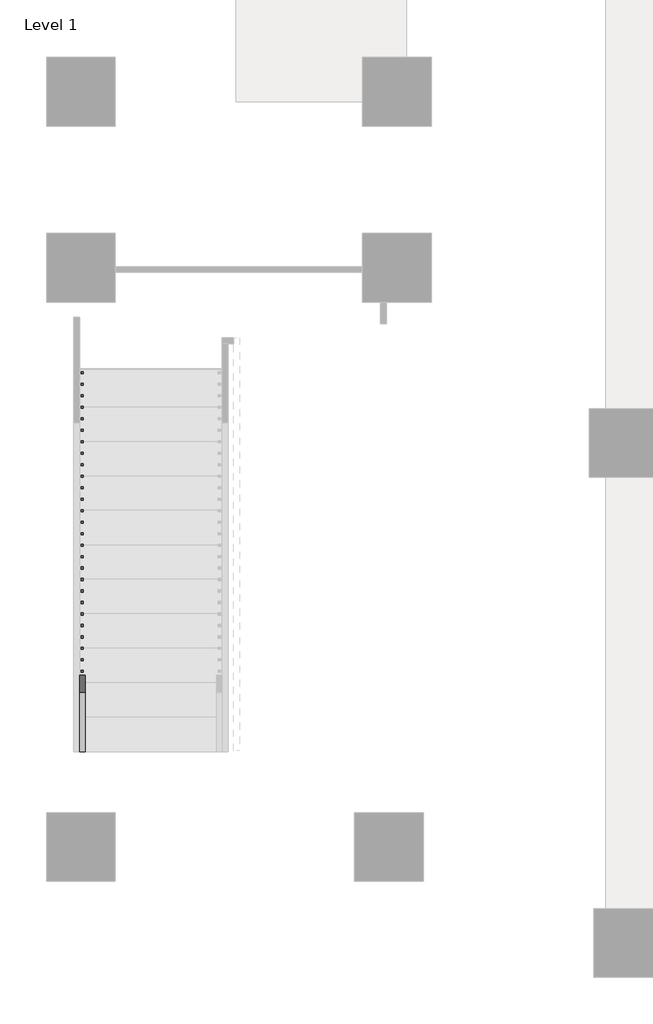
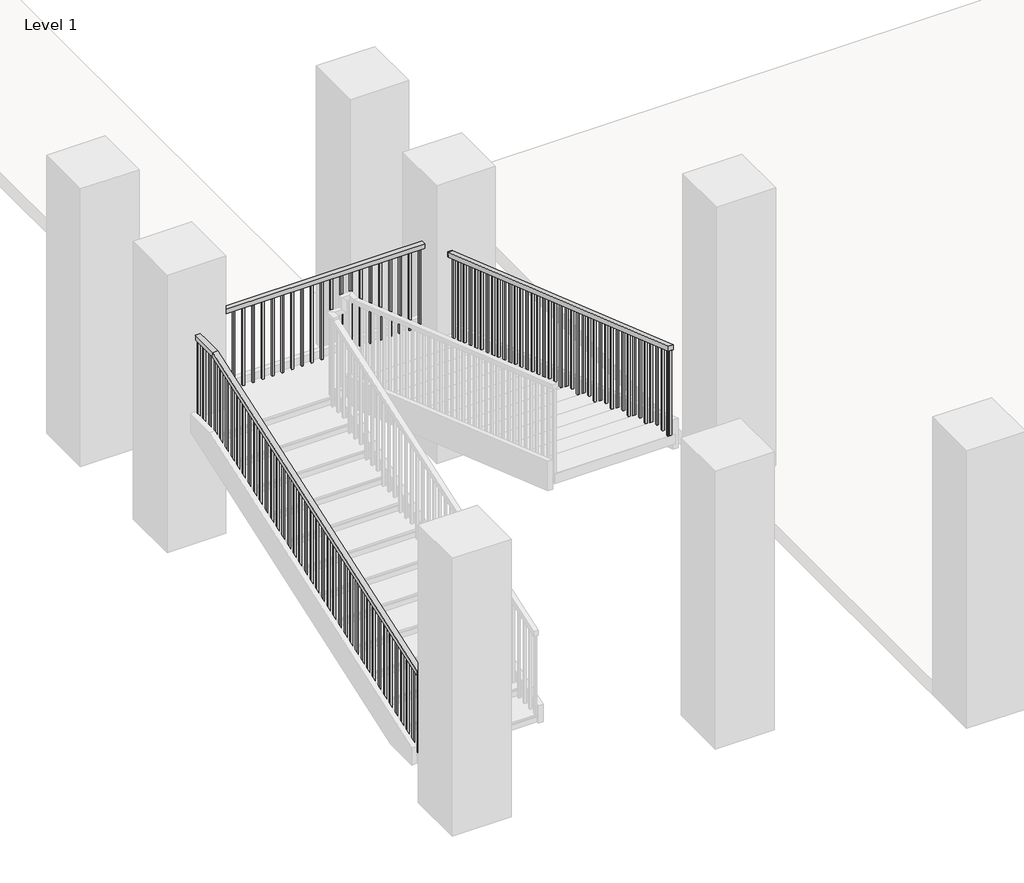
# One storey, part 4 of 6: 1 railing.
"""IFC4 building model written with IfcOpenShell, lengths in millimetres."""

from ifc_helpers import new_model, si_unit, frame, origin, place, context, project, spatial, polyline, outline, extrude, faceted_brep, element, save

model = new_model("IFC4")

# Units and contexts
model_context = context("Model", 3, world=origin())
ifc_project = project(units=[si_unit("LENGTHUNIT", "METRE", prefix="MILLI")], contexts=[model_context])

# Site, building, storey
site = spatial("IfcSite", under=ifc_project)
building = spatial("IfcBuilding", under=site)
storey = spatial("IfcBuildingStorey", under=building, Name="Level 1", Elevation=0.0)

# Railing
placement = place(None, origin())
element("IfcRailing", 1, ObjectType="Handrail - Rectangular", at=placement, inside=storey, context=model_context, shape_type="SolidModel", body=[
    faceted_brep([(-3857.687215, -9955.5916506, 1019.9076923), (-3857.687215, -9955.5916506, 966.1602476), (-3806.887215, -9955.5916506, 966.1602476), (-3806.887215, -9955.5916506, 1019.9076923), (-3857.687215, -6291.6416506, 2286.0), (-3857.687215, -6283.1120276, 2235.2), (-3806.887215, -6283.1120276, 2235.2), (-3806.887215, -6291.6416506, 2286.0), (-3857.687215, -5713.7916506, 2286.0), (-3857.687215, -5713.7916506, 2235.2), (-3806.887215, -5764.5916506, 2235.2), (-3806.887215, -5764.5916506, 2286.0), (-1190.687215, -5713.7916506, 2286.0), (-1190.687215, -5713.7916506, 2235.2), (-1241.487215, -5764.5916506, 2235.2), (-1241.487215, -5764.5916506, 2286.0), (-1190.687215, -5986.8416506, 2286.0), (-1190.687215, -5995.3852679, 2235.2), (-1241.487215, -5995.3852679, 2235.2), (-1241.487215, -5986.8416506, 2286.0), (-1190.687215, -9949.2416506, 3657.6), (-1241.487215, -9949.2416506, 3657.6), (-1241.487215, -9949.2416506, 3603.842594), (-1190.687215, -9949.2416506, 3603.842594)], [[[0, 1, 2, 3]], [[1, 0, 4, 5]], [[2, 1, 5, 6]], [[3, 2, 6, 7]], [[0, 3, 7, 4]], [[5, 4, 8, 9]], [[6, 5, 9, 10]], [[7, 6, 10, 11]], [[4, 7, 11, 8]], [[9, 8, 12, 13]], [[10, 9, 13, 14]], [[11, 10, 14, 15]], [[8, 11, 15, 12]], [[13, 12, 16, 17]], [[14, 13, 17, 18]], [[15, 14, 18, 19]], [[12, 15, 19, 16]], [[20, 21, 22, 23]], [[17, 16, 20, 23]], [[18, 17, 23, 22]], [[19, 18, 22, 21]], [[16, 19, 21, 20]]]),
    extrude(outline(polyline([(-9895.2666506, 3585.1589402), (-9895.2666506, 2637.6923077), (-9914.3166506, 2637.6923077), (-9914.3166506, 3591.7531709), (-9895.2666506, 3585.1589402)])), frame((-1225.612215, 0.0, 0.0), z_axis=(1.0, 0.0, 0.0), x_axis=(0.0, 1.0, 0.0)), (0.0, 0.0, 1.0), 19.05),
    extrude(outline(polyline([(-9793.6666506, 3549.9897094), (-9793.6666506, 2637.6923077), (-9812.7166506, 2637.6923077), (-9812.7166506, 3556.5839402), (-9793.6666506, 3549.9897094)])), frame((-1225.612215, 0.0, 0.0), z_axis=(1.0, 0.0, 0.0), x_axis=(0.0, 1.0, 0.0)), (0.0, 0.0, 1.0), 19.05),
    extrude(outline(polyline([(-9692.0666506, 3514.8204786), (-9692.0666506, 2637.6923077), (-9711.1166506, 2637.6923077), (-9711.1166506, 3521.4147094), (-9692.0666506, 3514.8204786)])), frame((-1225.612215, 0.0, 0.0), z_axis=(1.0, 0.0, 0.0), x_axis=(0.0, 1.0, 0.0)), (0.0, 0.0, 1.0), 19.05),
    extrude(outline(polyline([(-9590.4666506, 3479.6512479), (-9590.4666506, 2532.1846154), (-9609.5166506, 2532.1846154), (-9609.5166506, 3486.2454786), (-9590.4666506, 3479.6512479)])), frame((-1225.612215, 0.0, 0.0), z_axis=(1.0, 0.0, 0.0), x_axis=(0.0, 1.0, 0.0)), (0.0, 0.0, 1.0), 19.05),
    extrude(outline(polyline([(-9488.8666506, 3444.4820171), (-9488.8666506, 2532.1846154), (-9507.9166506, 2532.1846154), (-9507.9166506, 3451.0762479), (-9488.8666506, 3444.4820171)])), frame((-1225.612215, 0.0, 0.0), z_axis=(1.0, 0.0, 0.0), x_axis=(0.0, 1.0, 0.0)), (0.0, 0.0, 1.0), 19.05),
    extrude(outline(polyline([(-9387.2666506, 3409.3127863), (-9387.2666506, 2532.1846154), (-9406.3166506, 2532.1846154), (-9406.3166506, 3415.9070171), (-9387.2666506, 3409.3127863)])), frame((-1225.612215, 0.0, 0.0), z_axis=(1.0, 0.0, 0.0), x_axis=(0.0, 1.0, 0.0)), (0.0, 0.0, 1.0), 19.05),
    extrude(outline(polyline([(-9285.6666506, 3374.1435556), (-9285.6666506, 2426.6769231), (-9304.7166506, 2426.6769231), (-9304.7166506, 3380.7377863), (-9285.6666506, 3374.1435556)])), frame((-1225.612215, 0.0, 0.0), z_axis=(1.0, 0.0, 0.0), x_axis=(0.0, 1.0, 0.0)), (0.0, 0.0, 1.0), 19.05),
    extrude(outline(polyline([(-9184.0666506, 3338.9743248), (-9184.0666506, 2426.6769231), (-9203.1166506, 2426.6769231), (-9203.1166506, 3345.5685556), (-9184.0666506, 3338.9743248)])), frame((-1225.612215, 0.0, 0.0), z_axis=(1.0, 0.0, 0.0), x_axis=(0.0, 1.0, 0.0)), (0.0, 0.0, 1.0), 19.05),
    extrude(outline(polyline([(-9082.4666506, 3303.805094), (-9082.4666506, 2426.6769231), (-9101.5166506, 2426.6769231), (-9101.5166506, 3310.3993248), (-9082.4666506, 3303.805094)])), frame((-1225.612215, 0.0, 0.0), z_axis=(1.0, 0.0, 0.0), x_axis=(0.0, 1.0, 0.0)), (0.0, 0.0, 1.0), 19.05),
    extrude(outline(polyline([(-8980.8666506, 3268.6358632), (-8980.8666506, 2321.1692308), (-8999.9166506, 2321.1692308), (-8999.9166506, 3275.230094), (-8980.8666506, 3268.6358632)])), frame((-1225.612215, 0.0, 0.0), z_axis=(1.0, 0.0, 0.0), x_axis=(0.0, 1.0, 0.0)), (0.0, 0.0, 1.0), 19.05),
    extrude(outline(polyline([(-8879.2666506, 3233.4666325), (-8879.2666506, 2321.1692308), (-8898.3166506, 2321.1692308), (-8898.3166506, 3240.0608632), (-8879.2666506, 3233.4666325)])), frame((-1225.612215, 0.0, 0.0), z_axis=(1.0, 0.0, 0.0), x_axis=(0.0, 1.0, 0.0)), (0.0, 0.0, 1.0), 19.05),
    extrude(outline(polyline([(-8777.6666506, 3198.2974017), (-8777.6666506, 2321.1692308), (-8796.7166506, 2321.1692308), (-8796.7166506, 3204.8916325), (-8777.6666506, 3198.2974017)])), frame((-1225.612215, 0.0, 0.0), z_axis=(1.0, 0.0, 0.0), x_axis=(0.0, 1.0, 0.0)), (0.0, 0.0, 1.0), 19.05),
    extrude(outline(polyline([(-8676.0666506, 3163.1281709), (-8676.0666506, 2215.6615385), (-8695.1166506, 2215.6615385), (-8695.1166506, 3169.7224017), (-8676.0666506, 3163.1281709)])), frame((-1225.612215, 0.0, 0.0), z_axis=(1.0, 0.0, 0.0), x_axis=(0.0, 1.0, 0.0)), (0.0, 0.0, 1.0), 19.05),
    extrude(outline(polyline([(-8574.4666506, 3127.9589402), (-8574.4666506, 2215.6615385), (-8593.5166506, 2215.6615385), (-8593.5166506, 3134.5531709), (-8574.4666506, 3127.9589402)])), frame((-1225.612215, 0.0, 0.0), z_axis=(1.0, 0.0, 0.0), x_axis=(0.0, 1.0, 0.0)), (0.0, 0.0, 1.0), 19.05),
    extrude(outline(polyline([(-8472.8666506, 3092.7897094), (-8472.8666506, 2215.6615385), (-8491.9166506, 2215.6615385), (-8491.9166506, 3099.3839402), (-8472.8666506, 3092.7897094)])), frame((-1225.612215, 0.0, 0.0), z_axis=(1.0, 0.0, 0.0), x_axis=(0.0, 1.0, 0.0)), (0.0, 0.0, 1.0), 19.05),
    extrude(outline(polyline([(-8371.2666506, 3057.6204786), (-8371.2666506, 2110.1538462), (-8390.3166506, 2110.1538462), (-8390.3166506, 3064.2147094), (-8371.2666506, 3057.6204786)])), frame((-1225.612215, 0.0, 0.0), z_axis=(1.0, 0.0, 0.0), x_axis=(0.0, 1.0, 0.0)), (0.0, 0.0, 1.0), 19.05),
    extrude(outline(polyline([(-8269.6666506, 3022.4512479), (-8269.6666506, 2110.1538462), (-8288.7166506, 2110.1538462), (-8288.7166506, 3029.0454786), (-8269.6666506, 3022.4512479)])), frame((-1225.612215, 0.0, 0.0), z_axis=(1.0, 0.0, 0.0), x_axis=(0.0, 1.0, 0.0)), (0.0, 0.0, 1.0), 19.05),
    extrude(outline(polyline([(-8168.0666506, 2987.2820171), (-8168.0666506, 2110.1538462), (-8187.1166506, 2110.1538462), (-8187.1166506, 2993.8762479), (-8168.0666506, 2987.2820171)])), frame((-1225.612215, 0.0, 0.0), z_axis=(1.0, 0.0, 0.0), x_axis=(0.0, 1.0, 0.0)), (0.0, 0.0, 1.0), 19.05),
    extrude(outline(polyline([(-8066.4666506, 2952.1127863), (-8066.4666506, 2004.6461538), (-8085.5166506, 2004.6461538), (-8085.5166506, 2958.7070171), (-8066.4666506, 2952.1127863)])), frame((-1225.612215, 0.0, 0.0), z_axis=(1.0, 0.0, 0.0), x_axis=(0.0, 1.0, 0.0)), (0.0, 0.0, 1.0), 19.05),
    extrude(outline(polyline([(-7964.8666506, 2916.9435556), (-7964.8666506, 2004.6461538), (-7983.9166506, 2004.6461538), (-7983.9166506, 2923.5377863), (-7964.8666506, 2916.9435556)])), frame((-1225.612215, 0.0, 0.0), z_axis=(1.0, 0.0, 0.0), x_axis=(0.0, 1.0, 0.0)), (0.0, 0.0, 1.0), 19.05),
    extrude(outline(polyline([(-7863.2666506, 2881.7743248), (-7863.2666506, 2004.6461538), (-7882.3166506, 2004.6461538), (-7882.3166506, 2888.3685556), (-7863.2666506, 2881.7743248)])), frame((-1225.612215, 0.0, 0.0), z_axis=(1.0, 0.0, 0.0), x_axis=(0.0, 1.0, 0.0)), (0.0, 0.0, 1.0), 19.05),
    extrude(outline(polyline([(-7761.6666506, 2846.605094), (-7761.6666506, 1899.1384615), (-7780.7166506, 1899.1384615), (-7780.7166506, 2853.1993248), (-7761.6666506, 2846.605094)])), frame((-1225.612215, 0.0, 0.0), z_axis=(1.0, 0.0, 0.0), x_axis=(0.0, 1.0, 0.0)), (0.0, 0.0, 1.0), 19.05),
    extrude(outline(polyline([(-7660.0666506, 2811.4358632), (-7660.0666506, 1899.1384615), (-7679.1166506, 1899.1384615), (-7679.1166506, 2818.030094), (-7660.0666506, 2811.4358632)])), frame((-1225.612215, 0.0, 0.0), z_axis=(1.0, 0.0, 0.0), x_axis=(0.0, 1.0, 0.0)), (0.0, 0.0, 1.0), 19.05),
    extrude(outline(polyline([(-7558.4666506, 2776.2666325), (-7558.4666506, 1899.1384615), (-7577.5166506, 1899.1384615), (-7577.5166506, 2782.8608632), (-7558.4666506, 2776.2666325)])), frame((-1225.612215, 0.0, 0.0), z_axis=(1.0, 0.0, 0.0), x_axis=(0.0, 1.0, 0.0)), (0.0, 0.0, 1.0), 19.05),
    extrude(outline(polyline([(-7456.8666506, 2741.0974017), (-7456.8666506, 1793.6307692), (-7475.9166506, 1793.6307692), (-7475.9166506, 2747.6916325), (-7456.8666506, 2741.0974017)])), frame((-1225.612215, 0.0, 0.0), z_axis=(1.0, 0.0, 0.0), x_axis=(0.0, 1.0, 0.0)), (0.0, 0.0, 1.0), 19.05),
    extrude(outline(polyline([(-7355.2666506, 2705.9281709), (-7355.2666506, 1793.6307692), (-7374.3166506, 1793.6307692), (-7374.3166506, 2712.5224017), (-7355.2666506, 2705.9281709)])), frame((-1225.612215, 0.0, 0.0), z_axis=(1.0, 0.0, 0.0), x_axis=(0.0, 1.0, 0.0)), (0.0, 0.0, 1.0), 19.05),
    extrude(outline(polyline([(-7253.6666506, 2670.7589402), (-7253.6666506, 1793.6307692), (-7272.7166506, 1793.6307692), (-7272.7166506, 2677.3531709), (-7253.6666506, 2670.7589402)])), frame((-1225.612215, 0.0, 0.0), z_axis=(1.0, 0.0, 0.0), x_axis=(0.0, 1.0, 0.0)), (0.0, 0.0, 1.0), 19.05),
    extrude(outline(polyline([(-7152.0666506, 2635.5897094), (-7152.0666506, 1688.1230769), (-7171.1166506, 1688.1230769), (-7171.1166506, 2642.1839402), (-7152.0666506, 2635.5897094)])), frame((-1225.612215, 0.0, 0.0), z_axis=(1.0, 0.0, 0.0), x_axis=(0.0, 1.0, 0.0)), (0.0, 0.0, 1.0), 19.05),
    extrude(outline(polyline([(-7050.4666506, 2600.4204786), (-7050.4666506, 1688.1230769), (-7069.5166506, 1688.1230769), (-7069.5166506, 2607.0147094), (-7050.4666506, 2600.4204786)])), frame((-1225.612215, 0.0, 0.0), z_axis=(1.0, 0.0, 0.0), x_axis=(0.0, 1.0, 0.0)), (0.0, 0.0, 1.0), 19.05),
    extrude(outline(polyline([(-6948.8666506, 2565.2512479), (-6948.8666506, 1688.1230769), (-6967.9166506, 1688.1230769), (-6967.9166506, 2571.8454786), (-6948.8666506, 2565.2512479)])), frame((-1225.612215, 0.0, 0.0), z_axis=(1.0, 0.0, 0.0), x_axis=(0.0, 1.0, 0.0)), (0.0, 0.0, 1.0), 19.05),
    extrude(outline(polyline([(-6847.2666506, 2530.0820171), (-6847.2666506, 1582.6153846), (-6866.3166506, 1582.6153846), (-6866.3166506, 2536.6762479), (-6847.2666506, 2530.0820171)])), frame((-1225.612215, 0.0, 0.0), z_axis=(1.0, 0.0, 0.0), x_axis=(0.0, 1.0, 0.0)), (0.0, 0.0, 1.0), 19.05),
    extrude(outline(polyline([(-6745.6666506, 2494.9127863), (-6745.6666506, 1582.6153846), (-6764.7166506, 1582.6153846), (-6764.7166506, 2501.5070171), (-6745.6666506, 2494.9127863)])), frame((-1225.612215, 0.0, 0.0), z_axis=(1.0, 0.0, 0.0), x_axis=(0.0, 1.0, 0.0)), (0.0, 0.0, 1.0), 19.05),
    extrude(outline(polyline([(-6644.0666506, 2459.7435556), (-6644.0666506, 1582.6153846), (-6663.1166506, 1582.6153846), (-6663.1166506, 2466.3377863), (-6644.0666506, 2459.7435556)])), frame((-1225.612215, 0.0, 0.0), z_axis=(1.0, 0.0, 0.0), x_axis=(0.0, 1.0, 0.0)), (0.0, 0.0, 1.0), 19.05),
    extrude(outline(polyline([(-6542.4666506, 2424.5743248), (-6542.4666506, 1477.1076923), (-6561.5166506, 1477.1076923), (-6561.5166506, 2431.1685556), (-6542.4666506, 2424.5743248)])), frame((-1225.612215, 0.0, 0.0), z_axis=(1.0, 0.0, 0.0), x_axis=(0.0, 1.0, 0.0)), (0.0, 0.0, 1.0), 19.05),
    extrude(outline(polyline([(-6440.8666506, 2389.405094), (-6440.8666506, 1477.1076923), (-6459.9166506, 1477.1076923), (-6459.9166506, 2395.9993248), (-6440.8666506, 2389.405094)])), frame((-1225.612215, 0.0, 0.0), z_axis=(1.0, 0.0, 0.0), x_axis=(0.0, 1.0, 0.0)), (0.0, 0.0, 1.0), 19.05),
    extrude(outline(polyline([(-6339.2666506, 2354.2358632), (-6339.2666506, 1477.1076923), (-6358.3166506, 1477.1076923), (-6358.3166506, 2360.830094), (-6339.2666506, 2354.2358632)])), frame((-1225.612215, 0.0, 0.0), z_axis=(1.0, 0.0, 0.0), x_axis=(0.0, 1.0, 0.0)), (0.0, 0.0, 1.0), 19.05),
    extrude(outline(polyline([(-6237.6666506, 2319.0666325), (-6237.6666506, 1371.6), (-6256.7166506, 1371.6), (-6256.7166506, 2325.6608632), (-6237.6666506, 2319.0666325)])), frame((-1225.612215, 0.0, 0.0), z_axis=(1.0, 0.0, 0.0), x_axis=(0.0, 1.0, 0.0)), (0.0, 0.0, 1.0), 19.05),
    extrude(outline(polyline([(-6136.0666506, 2283.8974017), (-6136.0666506, 1371.6), (-6155.1166506, 1371.6), (-6155.1166506, 2290.4916325), (-6136.0666506, 2283.8974017)])), frame((-1225.612215, 0.0, 0.0), z_axis=(1.0, 0.0, 0.0), x_axis=(0.0, 1.0, 0.0)), (0.0, 0.0, 1.0), 19.05),
    extrude(outline(polyline([(-6034.4666506, 2248.7281709), (-6034.4666506, 1371.6), (-6053.5166506, 1371.6), (-6053.5166506, 2255.3224017), (-6034.4666506, 2248.7281709)])), frame((-1225.612215, 0.0, 0.0), z_axis=(1.0, 0.0, 0.0), x_axis=(0.0, 1.0, 0.0)), (0.0, 0.0, 1.0), 19.05),
    extrude(outline(polyline([(-1206.562215, -5932.8666506), (-1206.562215, -5951.9166506), (-1225.612215, -5951.9166506), (-1225.612215, -5932.8666506), (-1206.562215, -5932.8666506)])), frame((0.0, 0.0, 1371.6), z_axis=(0.0, 0.0, 1.0), x_axis=(1.0, 0.0, 0.0)), (0.0, 0.0, 1.0), 863.6),
    extrude(outline(polyline([(-1206.562215, -5831.2666506), (-1206.562215, -5850.3166506), (-1225.612215, -5850.3166506), (-1225.612215, -5831.2666506), (-1206.562215, -5831.2666506)])), frame((0.0, 0.0, 1371.6), z_axis=(0.0, 0.0, 1.0), x_axis=(1.0, 0.0, 0.0)), (0.0, 0.0, 1.0), 863.6),
    extrude(outline(polyline([(-1301.812215, -5729.6666506), (-1282.762215, -5729.6666506), (-1282.762215, -5748.7166506), (-1301.812215, -5748.7166506), (-1301.812215, -5729.6666506)])), frame((0.0, 0.0, 1371.6), z_axis=(0.0, 0.0, 1.0), x_axis=(1.0, 0.0, 0.0)), (0.0, 0.0, 1.0), 863.6),
    extrude(outline(polyline([(-1403.412215, -5729.6666506), (-1384.362215, -5729.6666506), (-1384.362215, -5748.7166506), (-1403.412215, -5748.7166506), (-1403.412215, -5729.6666506)])), frame((0.0, 0.0, 1371.6), z_axis=(0.0, 0.0, 1.0), x_axis=(1.0, 0.0, 0.0)), (0.0, 0.0, 1.0), 863.6),
    extrude(outline(polyline([(-1505.012215, -5729.6666506), (-1485.962215, -5729.6666506), (-1485.962215, -5748.7166506), (-1505.012215, -5748.7166506), (-1505.012215, -5729.6666506)])), frame((0.0, 0.0, 1371.6), z_axis=(0.0, 0.0, 1.0), x_axis=(1.0, 0.0, 0.0)), (0.0, 0.0, 1.0), 863.6),
    extrude(outline(polyline([(-1606.612215, -5729.6666506), (-1587.562215, -5729.6666506), (-1587.562215, -5748.7166506), (-1606.612215, -5748.7166506), (-1606.612215, -5729.6666506)])), frame((0.0, 0.0, 1371.6), z_axis=(0.0, 0.0, 1.0), x_axis=(1.0, 0.0, 0.0)), (0.0, 0.0, 1.0), 863.6),
    extrude(outline(polyline([(-1708.212215, -5729.6666506), (-1689.162215, -5729.6666506), (-1689.162215, -5748.7166506), (-1708.212215, -5748.7166506), (-1708.212215, -5729.6666506)])), frame((0.0, 0.0, 1371.6), z_axis=(0.0, 0.0, 1.0), x_axis=(1.0, 0.0, 0.0)), (0.0, 0.0, 1.0), 863.6),
    extrude(outline(polyline([(-1809.812215, -5729.6666506), (-1790.762215, -5729.6666506), (-1790.762215, -5748.7166506), (-1809.812215, -5748.7166506), (-1809.812215, -5729.6666506)])), frame((0.0, 0.0, 1371.6), z_axis=(0.0, 0.0, 1.0), x_axis=(1.0, 0.0, 0.0)), (0.0, 0.0, 1.0), 863.6),
    extrude(outline(polyline([(-1911.412215, -5729.6666506), (-1892.362215, -5729.6666506), (-1892.362215, -5748.7166506), (-1911.412215, -5748.7166506), (-1911.412215, -5729.6666506)])), frame((0.0, 0.0, 1371.6), z_axis=(0.0, 0.0, 1.0), x_axis=(1.0, 0.0, 0.0)), (0.0, 0.0, 1.0), 863.6),
    extrude(outline(polyline([(-2013.012215, -5729.6666506), (-1993.962215, -5729.6666506), (-1993.962215, -5748.7166506), (-2013.012215, -5748.7166506), (-2013.012215, -5729.6666506)])), frame((0.0, 0.0, 1371.6), z_axis=(0.0, 0.0, 1.0), x_axis=(1.0, 0.0, 0.0)), (0.0, 0.0, 1.0), 863.6),
    extrude(outline(polyline([(-2114.612215, -5729.6666506), (-2095.562215, -5729.6666506), (-2095.562215, -5748.7166506), (-2114.612215, -5748.7166506), (-2114.612215, -5729.6666506)])), frame((0.0, 0.0, 1371.6), z_axis=(0.0, 0.0, 1.0), x_axis=(1.0, 0.0, 0.0)), (0.0, 0.0, 1.0), 863.6),
    extrude(outline(polyline([(-2216.212215, -5729.6666506), (-2197.162215, -5729.6666506), (-2197.162215, -5748.7166506), (-2216.212215, -5748.7166506), (-2216.212215, -5729.6666506)])), frame((0.0, 0.0, 1371.6), z_axis=(0.0, 0.0, 1.0), x_axis=(1.0, 0.0, 0.0)), (0.0, 0.0, 1.0), 863.6),
    extrude(outline(polyline([(-2317.812215, -5729.6666506), (-2298.762215, -5729.6666506), (-2298.762215, -5748.7166506), (-2317.812215, -5748.7166506), (-2317.812215, -5729.6666506)])), frame((0.0, 0.0, 1371.6), z_axis=(0.0, 0.0, 1.0), x_axis=(1.0, 0.0, 0.0)), (0.0, 0.0, 1.0), 863.6),
    extrude(outline(polyline([(-2419.412215, -5729.6666506), (-2400.362215, -5729.6666506), (-2400.362215, -5748.7166506), (-2419.412215, -5748.7166506), (-2419.412215, -5729.6666506)])), frame((0.0, 0.0, 1371.6), z_axis=(0.0, 0.0, 1.0), x_axis=(1.0, 0.0, 0.0)), (0.0, 0.0, 1.0), 863.6),
    extrude(outline(polyline([(-2521.012215, -5729.6666506), (-2501.962215, -5729.6666506), (-2501.962215, -5748.7166506), (-2521.012215, -5748.7166506), (-2521.012215, -5729.6666506)])), frame((0.0, 0.0, 1371.6), z_axis=(0.0, 0.0, 1.0), x_axis=(1.0, 0.0, 0.0)), (0.0, 0.0, 1.0), 863.6),
    extrude(outline(polyline([(-2622.612215, -5729.6666506), (-2603.562215, -5729.6666506), (-2603.562215, -5748.7166506), (-2622.612215, -5748.7166506), (-2622.612215, -5729.6666506)])), frame((0.0, 0.0, 1371.6), z_axis=(0.0, 0.0, 1.0), x_axis=(1.0, 0.0, 0.0)), (0.0, 0.0, 1.0), 863.6),
    extrude(outline(polyline([(-2724.212215, -5729.6666506), (-2705.162215, -5729.6666506), (-2705.162215, -5748.7166506), (-2724.212215, -5748.7166506), (-2724.212215, -5729.6666506)])), frame((0.0, 0.0, 1371.6), z_axis=(0.0, 0.0, 1.0), x_axis=(1.0, 0.0, 0.0)), (0.0, 0.0, 1.0), 863.6),
    extrude(outline(polyline([(-2825.812215, -5729.6666506), (-2806.762215, -5729.6666506), (-2806.762215, -5748.7166506), (-2825.812215, -5748.7166506), (-2825.812215, -5729.6666506)])), frame((0.0, 0.0, 1371.6), z_axis=(0.0, 0.0, 1.0), x_axis=(1.0, 0.0, 0.0)), (0.0, 0.0, 1.0), 863.6),
    extrude(outline(polyline([(-2927.412215, -5729.6666506), (-2908.362215, -5729.6666506), (-2908.362215, -5748.7166506), (-2927.412215, -5748.7166506), (-2927.412215, -5729.6666506)])), frame((0.0, 0.0, 1371.6), z_axis=(0.0, 0.0, 1.0), x_axis=(1.0, 0.0, 0.0)), (0.0, 0.0, 1.0), 863.6),
    extrude(outline(polyline([(-3029.012215, -5729.6666506), (-3009.962215, -5729.6666506), (-3009.962215, -5748.7166506), (-3029.012215, -5748.7166506), (-3029.012215, -5729.6666506)])), frame((0.0, 0.0, 1371.6), z_axis=(0.0, 0.0, 1.0), x_axis=(1.0, 0.0, 0.0)), (0.0, 0.0, 1.0), 863.6),
    extrude(outline(polyline([(-3130.612215, -5729.6666506), (-3111.562215, -5729.6666506), (-3111.562215, -5748.7166506), (-3130.612215, -5748.7166506), (-3130.612215, -5729.6666506)])), frame((0.0, 0.0, 1371.6), z_axis=(0.0, 0.0, 1.0), x_axis=(1.0, 0.0, 0.0)), (0.0, 0.0, 1.0), 863.6),
    extrude(outline(polyline([(-3232.212215, -5729.6666506), (-3213.162215, -5729.6666506), (-3213.162215, -5748.7166506), (-3232.212215, -5748.7166506), (-3232.212215, -5729.6666506)])), frame((0.0, 0.0, 1371.6), z_axis=(0.0, 0.0, 1.0), x_axis=(1.0, 0.0, 0.0)), (0.0, 0.0, 1.0), 863.6),
    extrude(outline(polyline([(-3333.812215, -5729.6666506), (-3314.762215, -5729.6666506), (-3314.762215, -5748.7166506), (-3333.812215, -5748.7166506), (-3333.812215, -5729.6666506)])), frame((0.0, 0.0, 1371.6), z_axis=(0.0, 0.0, 1.0), x_axis=(1.0, 0.0, 0.0)), (0.0, 0.0, 1.0), 863.6),
    extrude(outline(polyline([(-3435.412215, -5729.6666506), (-3416.362215, -5729.6666506), (-3416.362215, -5748.7166506), (-3435.412215, -5748.7166506), (-3435.412215, -5729.6666506)])), frame((0.0, 0.0, 1371.6), z_axis=(0.0, 0.0, 1.0), x_axis=(1.0, 0.0, 0.0)), (0.0, 0.0, 1.0), 863.6),
    extrude(outline(polyline([(-3537.012215, -5729.6666506), (-3517.962215, -5729.6666506), (-3517.962215, -5748.7166506), (-3537.012215, -5748.7166506), (-3537.012215, -5729.6666506)])), frame((0.0, 0.0, 1371.6), z_axis=(0.0, 0.0, 1.0), x_axis=(1.0, 0.0, 0.0)), (0.0, 0.0, 1.0), 863.6),
    extrude(outline(polyline([(-3638.612215, -5729.6666506), (-3619.562215, -5729.6666506), (-3619.562215, -5748.7166506), (-3638.612215, -5748.7166506), (-3638.612215, -5729.6666506)])), frame((0.0, 0.0, 1371.6), z_axis=(0.0, 0.0, 1.0), x_axis=(1.0, 0.0, 0.0)), (0.0, 0.0, 1.0), 863.6),
    extrude(outline(polyline([(-3740.212215, -5729.6666506), (-3721.162215, -5729.6666506), (-3721.162215, -5748.7166506), (-3740.212215, -5748.7166506), (-3740.212215, -5729.6666506)])), frame((0.0, 0.0, 1371.6), z_axis=(0.0, 0.0, 1.0), x_axis=(1.0, 0.0, 0.0)), (0.0, 0.0, 1.0), 863.6),
    extrude(outline(polyline([(-3841.812215, -5799.5166506), (-3841.812215, -5780.4666506), (-3822.762215, -5780.4666506), (-3822.762215, -5799.5166506), (-3841.812215, -5799.5166506)])), frame((0.0, 0.0, 1371.6), z_axis=(0.0, 0.0, 1.0), x_axis=(1.0, 0.0, 0.0)), (0.0, 0.0, 1.0), 863.6),
    extrude(outline(polyline([(-3841.812215, -5901.1166506), (-3841.812215, -5882.0666506), (-3822.762215, -5882.0666506), (-3822.762215, -5901.1166506), (-3841.812215, -5901.1166506)])), frame((0.0, 0.0, 1371.6), z_axis=(0.0, 0.0, 1.0), x_axis=(1.0, 0.0, 0.0)), (0.0, 0.0, 1.0), 863.6),
    extrude(outline(polyline([(-3841.812215, -6002.7166506), (-3841.812215, -5983.6666506), (-3822.762215, -5983.6666506), (-3822.762215, -6002.7166506), (-3841.812215, -6002.7166506)])), frame((0.0, 0.0, 1371.6), z_axis=(0.0, 0.0, 1.0), x_axis=(1.0, 0.0, 0.0)), (0.0, 0.0, 1.0), 863.6),
    extrude(outline(polyline([(-3841.812215, -6104.3166506), (-3841.812215, -6085.2666506), (-3822.762215, -6085.2666506), (-3822.762215, -6104.3166506), (-3841.812215, -6104.3166506)])), frame((0.0, 0.0, 1371.6), z_axis=(0.0, 0.0, 1.0), x_axis=(1.0, 0.0, 0.0)), (0.0, 0.0, 1.0), 863.6),
    extrude(outline(polyline([(-3841.812215, -6205.9166506), (-3841.812215, -6186.8666506), (-3822.762215, -6186.8666506), (-3822.762215, -6205.9166506), (-3841.812215, -6205.9166506)])), frame((0.0, 0.0, 1371.6), z_axis=(0.0, 0.0, 1.0), x_axis=(1.0, 0.0, 0.0)), (0.0, 0.0, 1.0), 863.6),
    extrude(outline(polyline([(-6288.4666506, 2233.349689), (-6288.4666506, 1266.0923077), (-6307.5166506, 1266.0923077), (-6307.5166506, 2226.7668867), (-6288.4666506, 2233.349689)])), frame((-3841.812215, 0.0, 0.0), z_axis=(1.0, 0.0, 0.0), x_axis=(0.0, 1.0, 0.0)), (0.0, 0.0, 1.0), 19.05),
    extrude(outline(polyline([(-6390.0666506, 2198.2414101), (-6390.0666506, 1266.0923077), (-6409.1166506, 1266.0923077), (-6409.1166506, 2191.6586078), (-6390.0666506, 2198.2414101)])), frame((-3841.812215, 0.0, 0.0), z_axis=(1.0, 0.0, 0.0), x_axis=(0.0, 1.0, 0.0)), (0.0, 0.0, 1.0), 19.05),
    extrude(outline(polyline([(-6491.6666506, 2163.1331312), (-6491.6666506, 1266.0923077), (-6510.7166506, 1266.0923077), (-6510.7166506, 2156.5503289), (-6491.6666506, 2163.1331312)])), frame((-3841.812215, 0.0, 0.0), z_axis=(1.0, 0.0, 0.0), x_axis=(0.0, 1.0, 0.0)), (0.0, 0.0, 1.0), 19.05),
    extrude(outline(polyline([(-6593.2666506, 2128.0248523), (-6593.2666506, 1160.5846154), (-6612.3166506, 1160.5846154), (-6612.3166506, 2121.44205), (-6593.2666506, 2128.0248523)])), frame((-3841.812215, 0.0, 0.0), z_axis=(1.0, 0.0, 0.0), x_axis=(0.0, 1.0, 0.0)), (0.0, 0.0, 1.0), 19.05),
    extrude(outline(polyline([(-6694.8666506, 2092.9165734), (-6694.8666506, 1160.5846154), (-6713.9166506, 1160.5846154), (-6713.9166506, 2086.3337711), (-6694.8666506, 2092.9165734)])), frame((-3841.812215, 0.0, 0.0), z_axis=(1.0, 0.0, 0.0), x_axis=(0.0, 1.0, 0.0)), (0.0, 0.0, 1.0), 19.05),
    extrude(outline(polyline([(-6796.4666506, 2057.8082945), (-6796.4666506, 1160.5846154), (-6815.5166506, 1160.5846154), (-6815.5166506, 2051.2254922), (-6796.4666506, 2057.8082945)])), frame((-3841.812215, 0.0, 0.0), z_axis=(1.0, 0.0, 0.0), x_axis=(0.0, 1.0, 0.0)), (0.0, 0.0, 1.0), 19.05),
    extrude(outline(polyline([(-6898.0666506, 2022.7000156), (-6898.0666506, 1055.0769231), (-6917.1166506, 1055.0769231), (-6917.1166506, 2016.1172133), (-6898.0666506, 2022.7000156)])), frame((-3841.812215, 0.0, 0.0), z_axis=(1.0, 0.0, 0.0), x_axis=(0.0, 1.0, 0.0)), (0.0, 0.0, 1.0), 19.05),
    extrude(outline(polyline([(-6999.6666506, 1987.5917367), (-6999.6666506, 1055.0769231), (-7018.7166506, 1055.0769231), (-7018.7166506, 1981.0089344), (-6999.6666506, 1987.5917367)])), frame((-3841.812215, 0.0, 0.0), z_axis=(1.0, 0.0, 0.0), x_axis=(0.0, 1.0, 0.0)), (0.0, 0.0, 1.0), 19.05),
    extrude(outline(polyline([(-7101.2666506, 1952.4834578), (-7101.2666506, 1055.0769231), (-7120.3166506, 1055.0769231), (-7120.3166506, 1945.9006556), (-7101.2666506, 1952.4834578)])), frame((-3841.812215, 0.0, 0.0), z_axis=(1.0, 0.0, 0.0), x_axis=(0.0, 1.0, 0.0)), (0.0, 0.0, 1.0), 19.05),
    extrude(outline(polyline([(-7202.8666506, 1917.375179), (-7202.8666506, 949.5692308), (-7221.9166506, 949.5692308), (-7221.9166506, 1910.7923767), (-7202.8666506, 1917.375179)])), frame((-3841.812215, 0.0, 0.0), z_axis=(1.0, 0.0, 0.0), x_axis=(0.0, 1.0, 0.0)), (0.0, 0.0, 1.0), 19.05),
    extrude(outline(polyline([(-7304.4666506, 1882.2669001), (-7304.4666506, 949.5692308), (-7323.5166506, 949.5692308), (-7323.5166506, 1875.6840978), (-7304.4666506, 1882.2669001)])), frame((-3841.812215, 0.0, 0.0), z_axis=(1.0, 0.0, 0.0), x_axis=(0.0, 1.0, 0.0)), (0.0, 0.0, 1.0), 19.05),
    extrude(outline(polyline([(-7406.0666506, 1847.1586212), (-7406.0666506, 949.5692308), (-7425.1166506, 949.5692308), (-7425.1166506, 1840.5758189), (-7406.0666506, 1847.1586212)])), frame((-3841.812215, 0.0, 0.0), z_axis=(1.0, 0.0, 0.0), x_axis=(0.0, 1.0, 0.0)), (0.0, 0.0, 1.0), 19.05),
    extrude(outline(polyline([(-7507.6666506, 1812.0503423), (-7507.6666506, 844.0615385), (-7526.7166506, 844.0615385), (-7526.7166506, 1805.46754), (-7507.6666506, 1812.0503423)])), frame((-3841.812215, 0.0, 0.0), z_axis=(1.0, 0.0, 0.0), x_axis=(0.0, 1.0, 0.0)), (0.0, 0.0, 1.0), 19.05),
    extrude(outline(polyline([(-7609.2666506, 1776.9420634), (-7609.2666506, 844.0615385), (-7628.3166506, 844.0615385), (-7628.3166506, 1770.3592611), (-7609.2666506, 1776.9420634)])), frame((-3841.812215, 0.0, 0.0), z_axis=(1.0, 0.0, 0.0), x_axis=(0.0, 1.0, 0.0)), (0.0, 0.0, 1.0), 19.05),
    extrude(outline(polyline([(-7710.8666506, 1741.8337845), (-7710.8666506, 844.0615385), (-7729.9166506, 844.0615385), (-7729.9166506, 1735.2509822), (-7710.8666506, 1741.8337845)])), frame((-3841.812215, 0.0, 0.0), z_axis=(1.0, 0.0, 0.0), x_axis=(0.0, 1.0, 0.0)), (0.0, 0.0, 1.0), 19.05),
    extrude(outline(polyline([(-7812.4666506, 1706.7255056), (-7812.4666506, 738.5538462), (-7831.5166506, 738.5538462), (-7831.5166506, 1700.1427033), (-7812.4666506, 1706.7255056)])), frame((-3841.812215, 0.0, 0.0), z_axis=(1.0, 0.0, 0.0), x_axis=(0.0, 1.0, 0.0)), (0.0, 0.0, 1.0), 19.05),
    extrude(outline(polyline([(-7914.0666506, 1671.6172267), (-7914.0666506, 738.5538462), (-7933.1166506, 738.5538462), (-7933.1166506, 1665.0344244), (-7914.0666506, 1671.6172267)])), frame((-3841.812215, 0.0, 0.0), z_axis=(1.0, 0.0, 0.0), x_axis=(0.0, 1.0, 0.0)), (0.0, 0.0, 1.0), 19.05),
    extrude(outline(polyline([(-8015.6666506, 1636.5089478), (-8015.6666506, 738.5538462), (-8034.7166506, 738.5538462), (-8034.7166506, 1629.9261455), (-8015.6666506, 1636.5089478)])), frame((-3841.812215, 0.0, 0.0), z_axis=(1.0, 0.0, 0.0), x_axis=(0.0, 1.0, 0.0)), (0.0, 0.0, 1.0), 19.05),
    extrude(outline(polyline([(-8117.2666506, 1601.4006689), (-8117.2666506, 633.0461538), (-8136.3166506, 633.0461538), (-8136.3166506, 1594.8178666), (-8117.2666506, 1601.4006689)])), frame((-3841.812215, 0.0, 0.0), z_axis=(1.0, 0.0, 0.0), x_axis=(0.0, 1.0, 0.0)), (0.0, 0.0, 1.0), 19.05),
    extrude(outline(polyline([(-8218.8666506, 1566.29239), (-8218.8666506, 633.0461538), (-8237.9166506, 633.0461538), (-8237.9166506, 1559.7095877), (-8218.8666506, 1566.29239)])), frame((-3841.812215, 0.0, 0.0), z_axis=(1.0, 0.0, 0.0), x_axis=(0.0, 1.0, 0.0)), (0.0, 0.0, 1.0), 19.05),
    extrude(outline(polyline([(-8320.4666506, 1531.1841111), (-8320.4666506, 633.0461538), (-8339.5166506, 633.0461538), (-8339.5166506, 1524.6013088), (-8320.4666506, 1531.1841111)])), frame((-3841.812215, 0.0, 0.0), z_axis=(1.0, 0.0, 0.0), x_axis=(0.0, 1.0, 0.0)), (0.0, 0.0, 1.0), 19.05),
    extrude(outline(polyline([(-8422.0666506, 1496.0758322), (-8422.0666506, 527.5384615), (-8441.1166506, 527.5384615), (-8441.1166506, 1489.4930299), (-8422.0666506, 1496.0758322)])), frame((-3841.812215, 0.0, 0.0), z_axis=(1.0, 0.0, 0.0), x_axis=(0.0, 1.0, 0.0)), (0.0, 0.0, 1.0), 19.05),
    extrude(outline(polyline([(-8523.6666506, 1460.9675533), (-8523.6666506, 527.5384615), (-8542.7166506, 527.5384615), (-8542.7166506, 1454.384751), (-8523.6666506, 1460.9675533)])), frame((-3841.812215, 0.0, 0.0), z_axis=(1.0, 0.0, 0.0), x_axis=(0.0, 1.0, 0.0)), (0.0, 0.0, 1.0), 19.05),
    extrude(outline(polyline([(-8625.2666506, 1425.8592744), (-8625.2666506, 527.5384615), (-8644.3166506, 527.5384615), (-8644.3166506, 1419.2764721), (-8625.2666506, 1425.8592744)])), frame((-3841.812215, 0.0, 0.0), z_axis=(1.0, 0.0, 0.0), x_axis=(0.0, 1.0, 0.0)), (0.0, 0.0, 1.0), 19.05),
    extrude(outline(polyline([(-8726.8666506, 1390.7509955), (-8726.8666506, 422.0307692), (-8745.9166506, 422.0307692), (-8745.9166506, 1384.1681932), (-8726.8666506, 1390.7509955)])), frame((-3841.812215, 0.0, 0.0), z_axis=(1.0, 0.0, 0.0), x_axis=(0.0, 1.0, 0.0)), (0.0, 0.0, 1.0), 19.05),
    extrude(outline(polyline([(-8828.4666506, 1355.6427166), (-8828.4666506, 422.0307692), (-8847.5166506, 422.0307692), (-8847.5166506, 1349.0599143), (-8828.4666506, 1355.6427166)])), frame((-3841.812215, 0.0, 0.0), z_axis=(1.0, 0.0, 0.0), x_axis=(0.0, 1.0, 0.0)), (0.0, 0.0, 1.0), 19.05),
    extrude(outline(polyline([(-8930.0666506, 1320.5344377), (-8930.0666506, 422.0307692), (-8949.1166506, 422.0307692), (-8949.1166506, 1313.9516354), (-8930.0666506, 1320.5344377)])), frame((-3841.812215, 0.0, 0.0), z_axis=(1.0, 0.0, 0.0), x_axis=(0.0, 1.0, 0.0)), (0.0, 0.0, 1.0), 19.05),
    extrude(outline(polyline([(-9031.6666506, 1285.4261588), (-9031.6666506, 316.5230769), (-9050.7166506, 316.5230769), (-9050.7166506, 1278.8433565), (-9031.6666506, 1285.4261588)])), frame((-3841.812215, 0.0, 0.0), z_axis=(1.0, 0.0, 0.0), x_axis=(0.0, 1.0, 0.0)), (0.0, 0.0, 1.0), 19.05),
    extrude(outline(polyline([(-9133.2666506, 1250.3178799), (-9133.2666506, 316.5230769), (-9152.3166506, 316.5230769), (-9152.3166506, 1243.7350776), (-9133.2666506, 1250.3178799)])), frame((-3841.812215, 0.0, 0.0), z_axis=(1.0, 0.0, 0.0), x_axis=(0.0, 1.0, 0.0)), (0.0, 0.0, 1.0), 19.05),
    extrude(outline(polyline([(-9234.8666506, 1215.209601), (-9234.8666506, 316.5230769), (-9253.9166506, 316.5230769), (-9253.9166506, 1208.6267987), (-9234.8666506, 1215.209601)])), frame((-3841.812215, 0.0, 0.0), z_axis=(1.0, 0.0, 0.0), x_axis=(0.0, 1.0, 0.0)), (0.0, 0.0, 1.0), 19.05),
    extrude(outline(polyline([(-9336.4666506, 1180.1013221), (-9336.4666506, 211.0153846), (-9355.5166506, 211.0153846), (-9355.5166506, 1173.5185198), (-9336.4666506, 1180.1013221)])), frame((-3841.812215, 0.0, 0.0), z_axis=(1.0, 0.0, 0.0), x_axis=(0.0, 1.0, 0.0)), (0.0, 0.0, 1.0), 19.05),
    extrude(outline(polyline([(-9438.0666506, 1144.9930432), (-9438.0666506, 211.0153846), (-9457.1166506, 211.0153846), (-9457.1166506, 1138.4102409), (-9438.0666506, 1144.9930432)])), frame((-3841.812215, 0.0, 0.0), z_axis=(1.0, 0.0, 0.0), x_axis=(0.0, 1.0, 0.0)), (0.0, 0.0, 1.0), 19.05),
    extrude(outline(polyline([(-9539.6666506, 1109.8847643), (-9539.6666506, 211.0153846), (-9558.7166506, 211.0153846), (-9558.7166506, 1103.301962), (-9539.6666506, 1109.8847643)])), frame((-3841.812215, 0.0, 0.0), z_axis=(1.0, 0.0, 0.0), x_axis=(0.0, 1.0, 0.0)), (0.0, 0.0, 1.0), 19.05),
    extrude(outline(polyline([(-9641.2666506, 1074.7764854), (-9641.2666506, 105.5076923), (-9660.3166506, 105.5076923), (-9660.3166506, 1068.1936831), (-9641.2666506, 1074.7764854)])), frame((-3841.812215, 0.0, 0.0), z_axis=(1.0, 0.0, 0.0), x_axis=(0.0, 1.0, 0.0)), (0.0, 0.0, 1.0), 19.05),
    extrude(outline(polyline([(-9742.8666506, 1039.6682065), (-9742.8666506, 105.5076923), (-9761.9166506, 105.5076923), (-9761.9166506, 1033.0854043), (-9742.8666506, 1039.6682065)])), frame((-3841.812215, 0.0, 0.0), z_axis=(1.0, 0.0, 0.0), x_axis=(0.0, 1.0, 0.0)), (0.0, 0.0, 1.0), 19.05),
    extrude(outline(polyline([(-9844.4666506, 1004.5599277), (-9844.4666506, 105.5076923), (-9863.5166506, 105.5076923), (-9863.5166506, 997.9771254), (-9844.4666506, 1004.5599277)])), frame((-3841.812215, 0.0, 0.0), z_axis=(1.0, 0.0, 0.0), x_axis=(0.0, 1.0, 0.0)), (0.0, 0.0, 1.0), 19.05),
    extrude(outline(polyline([(-1225.612215, -5729.6666506), (-1206.562215, -5729.6666506), (-1206.562215, -5748.7166506), (-1225.612215, -5748.7166506), (-1225.612215, -5729.6666506)])), frame((0.0, 0.0, 1371.6), z_axis=(0.0, 0.0, 1.0), x_axis=(1.0, 0.0, 0.0)), (0.0, 0.0, 1.0), 863.6),
    extrude(outline(polyline([(-3841.812215, -5748.7166506), (-3841.812215, -5729.6666506), (-3822.762215, -5729.6666506), (-3822.762215, -5748.7166506), (-3841.812215, -5748.7166506)])), frame((0.0, 0.0, 1371.6), z_axis=(0.0, 0.0, 1.0), x_axis=(1.0, 0.0, 0.0)), (0.0, 0.0, 1.0), 863.6),
    extrude(outline(polyline([(-9930.1916506, 3597.2483632), (-9930.1916506, 2637.6923077), (-9949.2416506, 2637.6923077), (-9949.2416506, 3603.842594), (-9930.1916506, 3597.2483632)])), frame((-1225.612215, 0.0, 0.0), z_axis=(1.0, 0.0, 0.0), x_axis=(0.0, 1.0, 0.0)), (0.0, 0.0, 1.0), 19.05),
    extrude(outline(polyline([(-9936.5416506, 972.7430499), (-9936.5416506, 105.5076923), (-9955.5916506, 105.5076923), (-9955.5916506, 966.1602476), (-9936.5416506, 972.7430499)])), frame((-3841.812215, 0.0, 0.0), z_axis=(1.0, 0.0, 0.0), x_axis=(0.0, 1.0, 0.0)), (0.0, 0.0, 1.0), 19.05),
])

save(model, "model.ifc")

# Revit data of these elements
# Type "Handrail - Rectangular"
#   Assembly Code = "C2010400"
#   built-in parameter 1008612 = 0.0416667 (stored number, unit not read)
#   built-in parameter 1008611 = 0.0416667 (stored number, unit not read)
#   built-in parameter 1008609 = 0.333333 (stored number, unit not read)
#   built-in parameter 1008604 = 0.166667 (stored number, unit not read)
#   built-in parameter 1008603 = 0.166667 (stored number, unit not read)
#   Railing Height = 3' - 0"
#   built-in parameter 1008630 = 2
#   built-in parameter 1008610 = 2
#   built-in parameter 1008618 = Baluster - Square : 3/4"
# Element 1 (IfcRailing, "Handrail - Rectangular")
#   Phase Created = New Construction
